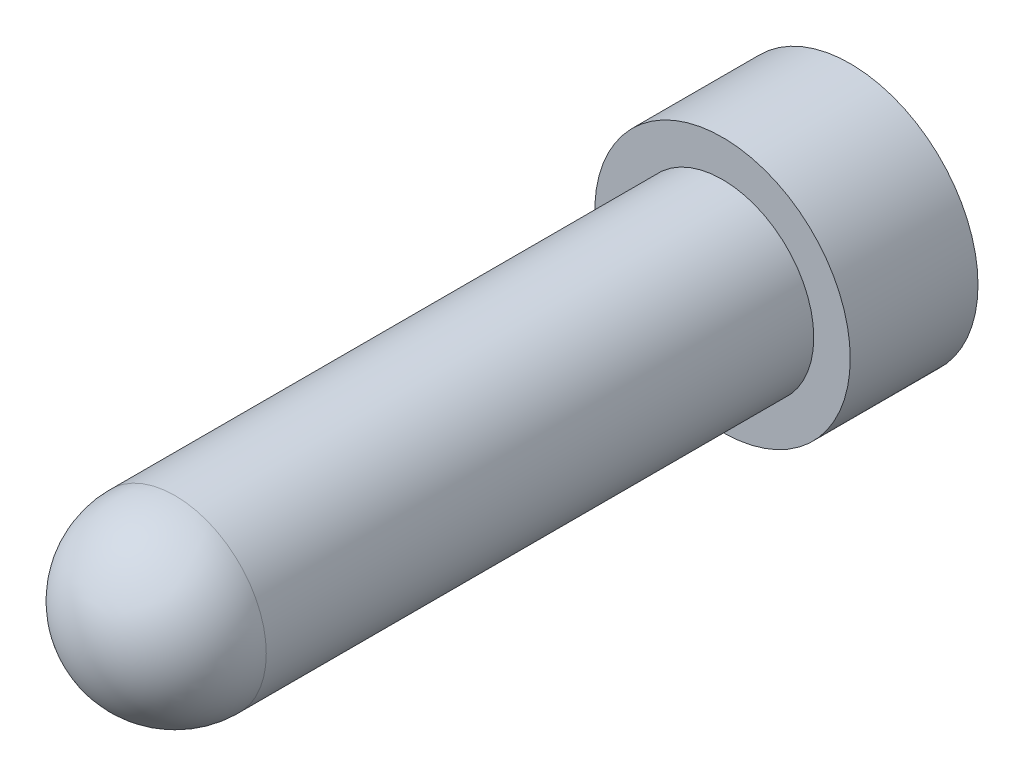
SolidWorks part; units mm, degrees
material "Plain Carbon Steel"
ref_plane "Front Plane" through (0, 0, 0) normal (0, 0, 1) x (1, 0, 0)
ref_plane "Top Plane" through (0, 0, 0) normal (0, 1, 0) x (1, 0, 0)
ref_plane "Right Plane" through (0, 0, 0) normal (1, 0, 0) x (0, 0, -1)
sketch "Head Profile Sketch" plane through (0, 0, 0) normal (0, 0, 1) x (1, 0, 0)
  line L0 (0, 30.6215) -> (0, -29.8292) construction
  line L1 (48.8835, 0) -> (-38.267, 0) construction
  circle A0 centre (0, 0) radius 7
  dimension "D1" = 14
extrude "Head Ø14x10" add sketch "Head Profile Sketch" along normal blind 7
sketch "Shank Profile Sketch" plane through (0, 0, 7) normal (0, 0, 1) x (1, 0, 0)
  circle A0 centre (0, 0) radius 5
  dimension "D1" = 10
extrude "Shank Ø10x35" add sketch "Shank Profile Sketch" along normal blind 35
fillet "Domed End R5" radius 5 1 edges at (5, 0, 42)
sketch "Hex Socket Sketch" plane through (0, 0, 0) normal (0, 0, -1) x (-1, 0, 0)
  line L1 (5.7735, 0) -> (2.8868, 5)
  line L2 (2.8868, 5) -> (-2.8868, 5)
  line L3 (-2.8868, 5) -> (-5.7735, 0)
  line L4 (-5.7735, 0) -> (-2.8868, -5)
  line L5 (-2.8868, -5) -> (2.8868, -5)
  line L6 (2.8868, -5) -> (5.7735, 0)
  circle A0 centre (0, 0) radius 5 construction
  dimension "D1" = 10
extrude "Hex Socket Cut 5 Deep" cut sketch "Hex Socket Sketch" against normal blind 5
